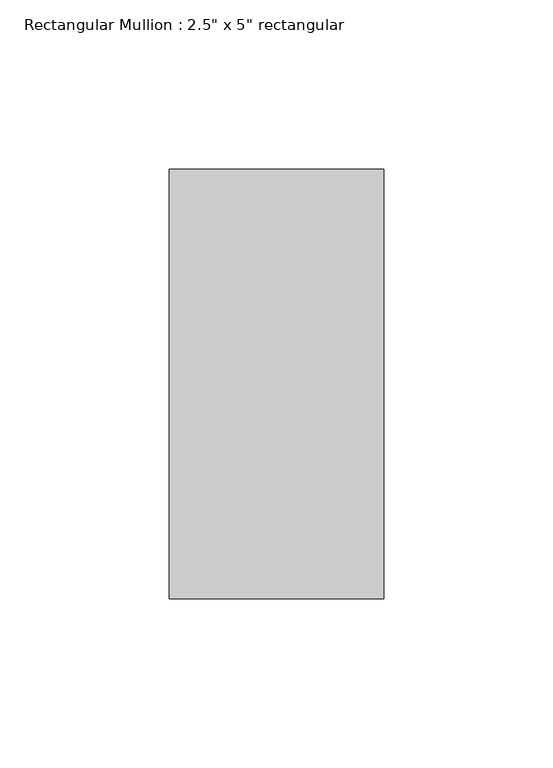
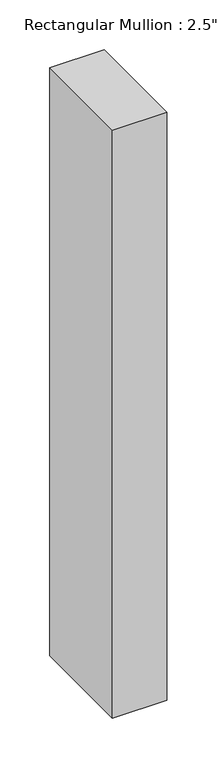
"""IFC4 building model written with IfcOpenShell, lengths in millimetres: member geometry."""

from ifc_helpers import new_model, si_unit, frame, origin, place, context, project, spatial, polyline, outline, extrude, source, transform, mapped, element, save


def member_93756e10(model_context):
    return source(origin(), model_context, "Body", "SweptSolid", [
        extrude(outline(polyline([(0.0, 63.5), (0.0, -63.5), (-63.5, -63.5), (-63.5, 63.5), (0.0, 63.5)])), frame((0.0, 0.0, -724.7301773), z_axis=(0.0, 0.0, 1.0), x_axis=(1.0, 0.0, 0.0)), (0.0, 0.0, 1.0), 724.7301773),
    ])


if __name__ == "__main__":
    model = new_model("IFC4")
    model_context = context("Model", 3, world=origin())
    ifc_project = project(units=[si_unit("LENGTHUNIT", "METRE", prefix="MILLI")], contexts=[model_context])
    site = spatial("IfcSite", under=ifc_project)
    building = spatial("IfcBuilding", under=site)
    placement = place(None, origin())
    member_shape = member_93756e10(model_context)
    element("IfcMember", 1, ObjectType="Rectangular Mullion : 2.5\" x 5\" rectangular", at=placement, inside=building, context=model_context, shape_type="MappedRepresentation", body=[
        mapped(member_shape, transform((0.0, 0.0, 0.0), x_axis=(1.0, 0.0, 0.0), y_axis=(0.0, 1.0, 0.0), z_axis=(0.0, 0.0, 1.0))),
    ])
    save(model, "model.ifc")

# Revit data of these elements
# Type "Rectangular Mullion : 2.5\" x 5\" rectangular"
#   built-in parameter 1007304 = 0.416667 (stored number, unit not read)
#   built-in parameter 1007301 = 0.104167 (stored number, unit not read)
#   built-in parameter 1007300 = 0.104167 (stored number, unit not read)
# Element 1 (IfcMember, "Rectangular Mullion : 2.5\" x 5\" rectangular")
#   Materials on its faces: "Aluminum"
# Materials
#   "Aluminum": class "Metal", colour RGB 247 247 247, transparency 0, Description = "Aluminum 6061", Cost = 0
